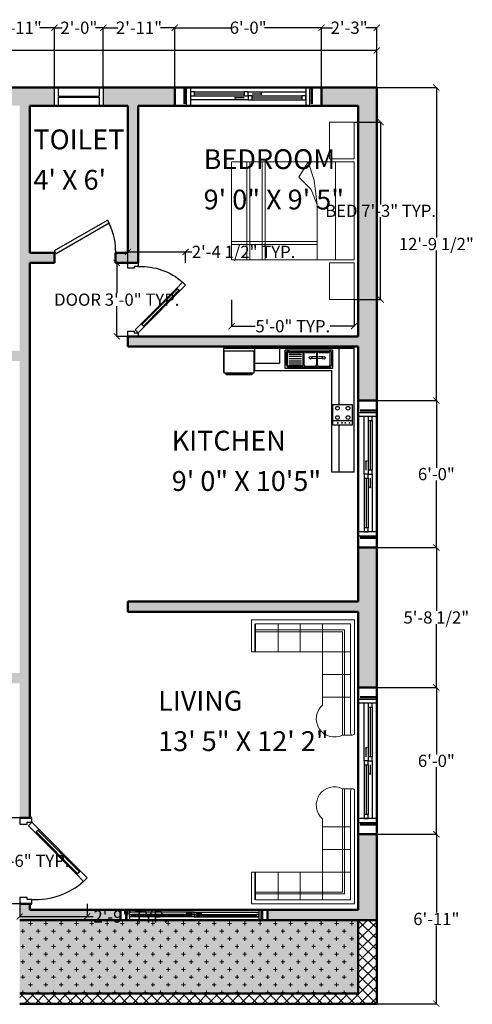
# Model space of a CAD drawing. Units: inches. Extents: x 2278 to 7495, y -71 to 1198.
# Tile 4 of 44: x 2542 to 2764, y 714 to 1197. Entities that reach past the tile are written whole.
import ezdxf

# ---------------------------------------------------------------- set-up
doc = ezdxf.new("R2010")
doc.units = ezdxf.units.IN
doc.header["$MEASUREMENT"] = 0
for name, color, linetype, lineweight in [('A-ANNO-DIMS', 2, 'Continuous', 18), ('A-AREA-IDEN', 3, 'Continuous', 18), ('A-Door', 3, 'Continuous', 25), ('A-FLOR-FIXT', 9, 'Continuous', 18), ('A-FURN', 8, 'Continuous', 18), ('A-Glaz', 4, 'Continuous', 25), ('A-Wall', 7, 'Continuous', 50), ('A-WALL-PATT', 8, 'Continuous', 18)]:
    doc.layers.add(name, color=color, linetype=linetype, lineweight=lineweight)
doc.layers.add('TEFRIŞ', color=11, linetype='Continuous')
doc.styles.get("Standard").update_dxf_attribs({"font": 'arial.ttf'})
doc.dimstyles.get("Standard").update_dxf_attribs({"dimtxt": 6, "dimasz": 3, "dimexe": 0.18, "dimexo": 0.0625, "dimgap": 0.09, "dimtad": 0, "dimtih": 1, "dimtoh": 1, "dimdec": 0, "dimzin": 0, "dimdsep": 46, "dimlunit": 3, "dimtxsty": 'Standard', "dimblk": 'ARCHTICK', "dimcen": 0.09, "dimadec": 0, "dimazin": 0, "dimtfac": 1, "dimtdec": 0, "dimtofl": 0, "dimtmove": 0, "dimatfit": 3, "dimfxl": 1, "dimtolj": 1, "dimtzin": 0, "dimarcsym": 0})

# ---------------------------------------------------------------- blocks, each defined once
blk = doc.blocks.new('A$C1DF4181C')
blk.add_lwpolyline([(120, 128), (460.7, 466.1), (432.5, 494.5), (91.8, 156.4)], close=True)
blk.add_arc((72.4, 128.7), 593.3, 357.23132, 41.49368)
at = {"layer": 'A-Door'}
for points in [[(517.5, 522.4), (460.7, 466.1), (432.5, 494.5), (489.3, 550.8)], [(35, 100), (0, 100), (0, 0), (50, 0), (50, 50), (50, 60), (35, 60)], [(63.2, 71.6), (120, 128), (91.8, 156.4), (35, 100)], [(665, 100), (665, 60), (650, 60), (650, 50), (650, 0), (700, 0), (700, 100)]]:
    blk.add_lwpolyline(points, close=True, dxfattribs=at)
at = {"layer": 'A-Glaz'}
blk.add_lwpolyline([(112.9, 135.1), (453.6, 473.2), (439.5, 487.4), (98.8, 149.3)], close=True, dxfattribs=at)
at = {"layer": 'A-Wall'}
for p, q in [((0, 0), (0, 100)), ((0, 100), (0, 0)), ((700, 0), (700, 100)), ((700, 0), (700, 100))]:
    blk.add_line(p, q, dxfattribs=at)
blk = doc.blocks.new('*U4')
for p, q in [((0, 0), (0, -6)), ((30, 0), (30, -6))]:
    blk.add_line(p, q)
blk.add_lwpolyline([(0, 0), (25.98, 15), (26.86, 13.48), (0.87, -1.52)], close=True)
blk.add_arc((0, 0), 30, 0, 30)
blk = doc.blocks.new('BED-160')
at = {"color": 0}
for p, q in [((-0.45, 2.35), (-0.45, 2.95)), ((-0.45, 2.95), (-0.05, 2.95)), ((-0.05, 2.95), (-0.05, 2.35)), ((-2.05, 2.3), (-0.05, 2.3)), ((-2.05, 0.7), (-2.05, 2.3)), ((-1.8, 0.7), (-1.8, 2.3)), ((-1.75, 0.7), (-1.75, 2.3)), ((-1.55, 0.7), (-1.55, 2.3)), ((-1.5, 0.7), (-1.5, 2.3)), ((-0.8, 2.3), (-0.95, 2.05)), ((-0.8, 2.3), (-0.7, 2)), ((-0.05, 2.35), (-0.45, 2.35)), ((-0.35, 0.7), (-0.35, 2.3)), ((-0.05, 2.3), (-0.05, 0.7)), ((-0.95, 2.05), (-0.75, 1.85)), ((-0.7, 2), (-0.65, 1.6)), ((-0.75, 1.85), (-0.65, 1.6)), ((-0.65, 1.6), (-0.65, 0.7)), ((-0.65, 1), (-2.05, 1)), ((-0.65, 0.95), (-2.05, 0.95)), ((-0.05, 0.7), (-2.05, 0.7)), ((-0.45, 0.65), (-0.05, 0.65)), ((-0.45, 0.05), (-0.45, 0.65)), ((-0.05, 0.65), (-0.05, 0.05)), ((-0.05, 0.05), (-0.45, 0.05))]:
    blk.add_line(p, q, dxfattribs=at)
blk = doc.blocks.new('A$C008029BD')
at = {"layer": 'TEFRIŞ', "ltscale": 0.05}
for p, q in [((0, 0), (0, -3.55)), ((3.37, 0), (0, 0)), ((3.37, 0), (3.37, -0.6)), ((1.522, -0.4), (0, -0.4)), ((3.37, -0.4), (2.083, -0.4)), ((0.05, -0.581), (0.05, -1.869)), ((0.05, -0.581), (0.55, -0.581)), ((0.086, -1.773), (0.086, -0.677)), ((0.096, -0.617), (0.454, -0.617)), ((0.099, -0.659), (0.457, -0.659)), ((0.113, -0.954), (0.113, -0.695)), ((0.493, -0.695), (0.493, -0.954)), ((0.514, -0.677), (0.514, -1.773)), ((0.55, -0.581), (0.55, -1.869)), ((0.6, -2.71), (0.6, -0.6)), ((3.37, -0.6), (0.6, -0.6)), ((0.096, -1.024), (0.454, -1.024)), ((0.457, -0.99), (0.099, -0.99)), ((0.11, -1.319), (0.11, -1.06)), ((0.228, -1.02), (0.227, -1.159)), ((0.23, -0.846), (0.229, -0.967)), ((0.28, -0.846), (0.277, -1.158)), ((0.49, -1.06), (0.49, -1.319)), ((0.454, -1.355), (0.096, -1.355)), ((0.096, -1.391), (0.454, -1.391)), ((0.11, -1.773), (0.11, -1.427)), ((0.154, -1.773), (0.154, -1.427)), ((0.214, -1.773), (0.214, -1.427)), ((0.274, -1.773), (0.274, -1.427)), ((0.334, -1.773), (0.334, -1.427)), ((0.39, -1.773), (0.39, -1.427)), ((0.444, -1.773), (0.444, -1.427)), ((0.49, -1.427), (0.49, -1.773)), ((0.55, -1.869), (0.05, -1.869)), ((0.454, -1.809), (0.096, -1.809)), ((0.454, -1.833), (0.096, -1.833)), ((0, -2.025), (0.4, -2.025)), ((0.4, -2.71), (0.4, -2.025)), ((0, -2.71), (0.6, -2.71)), ((0, -3.55), (0.65, -3.55))]:
    blk.add_line(p, q, dxfattribs=at)
at = {"layer": 'TEFRIŞ'}
blk.add_line((1.969, -0.05), (1.969, -0.572), dxfattribs=at)
at = {"layer": 'TEFRIŞ', "ltscale": 0.05}
for points in [[(1.522, -0.05), (2.083, -0.05), (2.083, -0.572), (1.522, -0.572)], [(0.67, -2.73), (0.67, -3.53), (0.07, -3.53), (0.07, -2.73)], [(0.72, -2.78), (0.72, -3.48), (0.67, -3.48), (0.67, -2.78)]]:
    blk.add_lwpolyline(points, close=True, dxfattribs=at)
at = {"layer": 'TEFRIŞ', "const_width": 0.025}
for points in [[(2.014, -0.123, 1), (2.039, -0.123, 1)], [(2.014, -0.236, 1), (2.039, -0.236, 1)], [(2.014, -0.327, 1), (2.039, -0.327, 1)], [(2.014, -0.44, 1), (2.039, -0.44, 1)]]:
    blk.add_lwpolyline(points, format="xyb", close=True, dxfattribs=at)
at = {"layer": 'TEFRIŞ', "ltscale": 0.05}
for centre, radius in [((1.628, -0.164), 0.0505), ((1.628, -0.45), 0.0505), ((0.255, -0.82), 0.036), ((0.252, -1.184), 0.036)]:
    blk.add_circle(centre, radius, dxfattribs=at)
at = {"layer": 'TEFRIŞ'}
for centre in [(1.88, -0.164), (1.88, -0.45)]:
    blk.add_circle(centre, 0.0505, dxfattribs=at)
at = {"layer": 'TEFRIŞ', "ltscale": 0.05}
for centre, radius, start, end in [((0.108, -0.649), 0.0351, 110.4976, 230.5777), ((0.118, -0.673), 0.023, 143.9853, 258.5157), ((0.454, -0.677), 0.06, 0, 90), ((0.457, -0.695), 0.036, 0, 90), ((0.115, -1.038), 0.023, 143.9853, 258.5157), ((0.118, -0.976), 0.023, 101.4843, 216.0147), ((0.454, -1.06), 0.036, 0, 90), ((0.457, -0.954), 0.036, 270, 0), ((0.115, -1.341), 0.023, 101.4843, 216.0147), ((0.454, -1.319), 0.036, 270, 0), ((0.115, -1.405), 0.023, 143.9853, 258.5157), ((0.454, -1.427), 0.036, 0, 90), ((0.108, -1.801), 0.0351, 129.4223, 249.5024), ((0.115, -1.796), 0.023, 101.4843, 216.0147), ((0.454, -1.773), 0.06, 270, 0), ((0.454, -1.773), 0.036, 270, 0)]:
    blk.add_arc(centre, radius, start, end, dxfattribs=at)
blk = doc.blocks.new('_ArchTick')
at = {"color": 0, "linetype": 'ByBlock', "const_width": 0.15}
blk.add_lwpolyline([(-0.5, -0.5), (0.5, 0.5)], dxfattribs=at)
blk = doc.blocks.new('*D18')
at = {"layer": 'A-ANNO-DIMS', "color": 0, "lineweight": -2, "transparency": 16777216}
for p, q in [((2313.87, 1163.53), (2313.87, 1181.72)), ((2313.87, 1181.54), (2504.98, 1181.54)), ((2716.87, 1181.54), (2525.76, 1181.54)), ((2716.87, 1163.53), (2716.87, 1181.72))]:
    blk.add_line(p, q, dxfattribs=at)
at = {"layer": 'Defpoints', "color": 0, "transparency": 16777216}
for p in [(2716.87, 1181.54), (2313.87, 1163.47), (2716.87, 1163.47)]:
    blk.add_point(p, dxfattribs=at)
at = {"layer": 'A-ANNO-DIMS', "color": 0, "lineweight": -2, "transparency": 16777216, "xscale": 3, "yscale": 3, "zscale": 3, "rotation": 180}
blk.add_blockref('_ArchTick', (2313.87, 1181.54), dxfattribs=at)
at = {"layer": 'A-ANNO-DIMS', "color": 0, "lineweight": -2, "transparency": 16777216, "xscale": 3, "yscale": 3, "zscale": 3}
blk.add_blockref('_ArchTick', (2716.87, 1181.54), dxfattribs=at)
at = {"layer": 'A-ANNO-DIMS', "color": 0, "transparency": 16777216, "insert": (2515.37, 1181.54), "char_height": 6, "attachment_point": 5}
blk.add_mtext('\\A1;33\'-7"', dxfattribs=at)
blk = doc.blocks.new('*D43')
at = {"layer": 'A-ANNO-DIMS', "color": 0, "lineweight": -2, "transparency": 16777216}
for p, q in [((2541.81, 805.47), (2535.39, 805.47)), ((2535.57, 805.47), (2535.57, 787.66)), ((2535.57, 763.47), (2535.57, 781.27)), ((2541.81, 763.47), (2535.39, 763.47))]:
    blk.add_line(p, q, dxfattribs=at)
at = {"layer": 'Defpoints', "color": 0, "transparency": 16777216}
for p in [(2541.87, 805.47), (2535.57, 763.47), (2541.87, 763.47)]:
    blk.add_point(p, dxfattribs=at)
at = {"layer": 'A-ANNO-DIMS', "color": 0, "lineweight": -2, "transparency": 16777216, "xscale": 3, "yscale": 3, "zscale": 3}
for p, rotation in [((2535.57, 805.47), 90), ((2535.57, 763.47), 270)]:
    blk.add_blockref('_ArchTick', p, dxfattribs=dict(at, rotation=rotation))
at = {"layer": 'A-ANNO-DIMS', "color": 0, "transparency": 16777216, "insert": (2535.57, 784.47), "char_height": 6, "attachment_point": 5}
blk.add_mtext('\\A1;DOOR 3\'-6" TYP.', dxfattribs=at)
blk = doc.blocks.new('*D44')
at = {"layer": 'A-ANNO-DIMS', "color": 0, "lineweight": -2, "transparency": 16777216}
for p, q in [((2541.87, 763.4), (2541.87, 756.99)), ((2574.92, 763.4), (2574.92, 756.99)), ((2541.87, 757.17), (2574.92, 757.17)), ((2574.92, 757.17), (2577.92, 757.17))]:
    blk.add_line(p, q, dxfattribs=at)
at = {"layer": 'Defpoints', "color": 0, "transparency": 16777216}
for p in [(2541.87, 763.47), (2574.92, 763.47), (2574.92, 757.17)]:
    blk.add_point(p, dxfattribs=at)
at = {"layer": 'A-ANNO-DIMS', "color": 0, "lineweight": -2, "transparency": 16777216, "xscale": 3, "yscale": 3, "zscale": 3, "rotation": 180}
blk.add_blockref('_ArchTick', (2541.87, 757.17), dxfattribs=at)
at = {"layer": 'A-ANNO-DIMS', "color": 0, "lineweight": -2, "transparency": 16777216, "xscale": 3, "yscale": 3, "zscale": 3}
blk.add_blockref('_ArchTick', (2574.92, 757.17), dxfattribs=at)
at = {"layer": 'A-ANNO-DIMS', "color": 0, "transparency": 16777216, "insert": (2596.35, 757.17), "char_height": 6, "attachment_point": 5}
blk.add_mtext('\\A1;2\'-9" TYP.', dxfattribs=at)
blk = doc.blocks.new('*D45')
at = {"layer": 'A-ANNO-DIMS', "color": 0, "lineweight": -2, "transparency": 16777216}
for p, q in [((2594.81, 1077.47), (2589.29, 1077.47)), ((2589.47, 1077.47), (2589.47, 1062.66)), ((2589.47, 1041.47), (2589.47, 1056.27)), ((2594.81, 1041.47), (2589.29, 1041.47))]:
    blk.add_line(p, q, dxfattribs=at)
at = {"layer": 'Defpoints', "color": 0, "transparency": 16777216}
for p in [(2589.47, 1077.47), (2594.87, 1077.47), (2594.87, 1041.47)]:
    blk.add_point(p, dxfattribs=at)
at = {"layer": 'A-ANNO-DIMS', "color": 0, "lineweight": -2, "transparency": 16777216, "xscale": 3, "yscale": 3, "zscale": 3}
for p, rotation in [((2589.47, 1077.47), 90), ((2589.47, 1041.47), 270)]:
    blk.add_blockref('_ArchTick', p, dxfattribs=dict(at, rotation=rotation))
at = {"layer": 'A-ANNO-DIMS', "color": 0, "transparency": 16777216, "insert": (2589.47, 1059.47), "char_height": 6, "attachment_point": 5}
blk.add_mtext('\\A1;DOOR 3\'-0" TYP.', dxfattribs=at)
blk = doc.blocks.new('*D46')
at = {"layer": 'A-ANNO-DIMS', "color": 0, "lineweight": -2, "transparency": 16777216}
for p, q in [((2594.87, 1077.53), (2594.87, 1083.05)), ((2594.87, 1082.87), (2623.2, 1082.87)), ((2623.2, 1077.53), (2623.2, 1083.05)), ((2623.2, 1082.87), (2626.2, 1082.87))]:
    blk.add_line(p, q, dxfattribs=at)
at = {"layer": 'Defpoints', "color": 0, "transparency": 16777216}
for p in [(2623.2, 1082.87), (2594.87, 1077.47), (2623.2, 1077.47)]:
    blk.add_point(p, dxfattribs=at)
at = {"layer": 'A-ANNO-DIMS', "color": 0, "lineweight": -2, "transparency": 16777216, "xscale": 3, "yscale": 3, "zscale": 3, "rotation": 180}
blk.add_blockref('_ArchTick', (2594.87, 1082.87), dxfattribs=at)
at = {"layer": 'A-ANNO-DIMS', "color": 0, "lineweight": -2, "transparency": 16777216, "xscale": 3, "yscale": 3, "zscale": 3}
blk.add_blockref('_ArchTick', (2623.2, 1082.87), dxfattribs=at)
at = {"layer": 'A-ANNO-DIMS', "color": 0, "transparency": 16777216, "insert": (2651.62, 1082.87), "char_height": 6, "attachment_point": 5}
blk.add_mtext('\\A1;2\'-4 1/2" TYP.', dxfattribs=at)
blk = doc.blocks.new('*D49')
at = {"layer": 'A-ANNO-DIMS', "color": 0, "lineweight": -2, "transparency": 16777216}
for p, q in [((2705.82, 1146.5), (2718.99, 1146.5)), ((2718.81, 1146.5), (2718.81, 1106.15)), ((2718.81, 1059.5), (2718.81, 1099.84)), ((2705.82, 1059.5), (2718.99, 1059.5))]:
    blk.add_line(p, q, dxfattribs=at)
at = {"layer": 'Defpoints', "color": 0, "transparency": 16777216}
for p in [(2705.76, 1146.5), (2718.81, 1146.5), (2705.76, 1059.5)]:
    blk.add_point(p, dxfattribs=at)
at = {"layer": 'A-ANNO-DIMS', "color": 0, "lineweight": -2, "transparency": 16777216, "xscale": 3, "yscale": 3, "zscale": 3}
for p, rotation in [((2718.81, 1146.5), 90), ((2718.81, 1059.5), 270)]:
    blk.add_blockref('_ArchTick', p, dxfattribs=dict(at, rotation=rotation))
at = {"layer": 'A-ANNO-DIMS', "color": 0, "transparency": 16777216, "insert": (2718.81, 1103), "char_height": 6, "attachment_point": 5}
blk.add_mtext('\\A1;BED 7\'-3" TYP.', dxfattribs=at)
blk = doc.blocks.new('*D50')
at = {"layer": 'A-ANNO-DIMS', "color": 0, "lineweight": -2, "transparency": 16777216}
for p, q in [((2645.76, 1059.43), (2645.76, 1046.27)), ((2705.76, 1059.43), (2705.76, 1046.27)), ((2645.76, 1046.45), (2657.38, 1046.45)), ((2705.76, 1046.45), (2694.14, 1046.45))]:
    blk.add_line(p, q, dxfattribs=at)
at = {"layer": 'Defpoints', "color": 0, "transparency": 16777216}
for p in [(2645.76, 1059.5), (2705.76, 1059.5), (2705.76, 1046.45)]:
    blk.add_point(p, dxfattribs=at)
at = {"layer": 'A-ANNO-DIMS', "color": 0, "lineweight": -2, "transparency": 16777216, "xscale": 3, "yscale": 3, "zscale": 3, "rotation": 180}
blk.add_blockref('_ArchTick', (2645.76, 1046.45), dxfattribs=at)
at = {"layer": 'A-ANNO-DIMS', "color": 0, "lineweight": -2, "transparency": 16777216, "xscale": 3, "yscale": 3, "zscale": 3}
blk.add_blockref('_ArchTick', (2705.76, 1046.45), dxfattribs=at)
at = {"layer": 'A-ANNO-DIMS', "color": 0, "transparency": 16777216, "insert": (2675.76, 1046.45), "char_height": 6, "attachment_point": 5}
blk.add_mtext('\\A1;5\'-0" TYP.', dxfattribs=at)
blk = doc.blocks.new('*D65')
at = {"layer": 'A-ANNO-DIMS', "color": 0, "lineweight": -2, "transparency": 16777216}
for p, q in [((2523.87, 1163.53), (2523.87, 1192.9)), ((2523.87, 1192.72), (2530.92, 1192.72)), ((2558.87, 1192.72), (2551.82, 1192.72)), ((2558.87, 1163.53), (2558.87, 1192.9))]:
    blk.add_line(p, q, dxfattribs=at)
at = {"layer": 'Defpoints', "color": 0, "transparency": 16777216}
for p in [(2558.87, 1192.72), (2523.87, 1163.47), (2558.87, 1163.47)]:
    blk.add_point(p, dxfattribs=at)
at = {"layer": 'A-ANNO-DIMS', "color": 0, "lineweight": -2, "transparency": 16777216, "xscale": 3, "yscale": 3, "zscale": 3, "rotation": 180}
blk.add_blockref('_ArchTick', (2523.87, 1192.72), dxfattribs=at)
at = {"layer": 'A-ANNO-DIMS', "color": 0, "lineweight": -2, "transparency": 16777216, "xscale": 3, "yscale": 3, "zscale": 3}
blk.add_blockref('_ArchTick', (2558.87, 1192.72), dxfattribs=at)
at = {"layer": 'A-ANNO-DIMS', "color": 0, "transparency": 16777216, "insert": (2541.37, 1192.72), "char_height": 6, "attachment_point": 5}
blk.add_mtext('\\A1;2\'-11"', dxfattribs=at)
blk = doc.blocks.new('*D66')
at = {"layer": 'A-ANNO-DIMS', "color": 0, "lineweight": -2, "transparency": 16777216}
for p, q in [((2558.87, 1163.53), (2558.87, 1192.9)), ((2558.87, 1192.72), (2562.75, 1192.72)), ((2582.87, 1192.72), (2578.99, 1192.72)), ((2582.87, 1163.53), (2582.87, 1192.9))]:
    blk.add_line(p, q, dxfattribs=at)
at = {"layer": 'Defpoints', "color": 0, "transparency": 16777216}
for p in [(2582.87, 1192.72), (2558.87, 1163.47), (2582.87, 1163.47)]:
    blk.add_point(p, dxfattribs=at)
at = {"layer": 'A-ANNO-DIMS', "color": 0, "lineweight": -2, "transparency": 16777216, "xscale": 3, "yscale": 3, "zscale": 3, "rotation": 180}
blk.add_blockref('_ArchTick', (2558.87, 1192.72), dxfattribs=at)
at = {"layer": 'A-ANNO-DIMS', "color": 0, "lineweight": -2, "transparency": 16777216, "xscale": 3, "yscale": 3, "zscale": 3}
blk.add_blockref('_ArchTick', (2582.87, 1192.72), dxfattribs=at)
at = {"layer": 'A-ANNO-DIMS', "color": 0, "transparency": 16777216, "insert": (2570.87, 1192.72), "char_height": 6, "attachment_point": 5}
blk.add_mtext('\\A1;2\'-0"', dxfattribs=at)
blk = doc.blocks.new('*D67')
at = {"layer": 'A-ANNO-DIMS', "color": 0, "lineweight": -2, "transparency": 16777216}
for p, q in [((2582.87, 1163.53), (2582.87, 1192.9)), ((2582.87, 1192.72), (2589.92, 1192.72)), ((2617.87, 1192.72), (2610.82, 1192.72)), ((2617.87, 1163.53), (2617.87, 1192.9))]:
    blk.add_line(p, q, dxfattribs=at)
at = {"layer": 'Defpoints', "color": 0, "transparency": 16777216}
for p in [(2617.87, 1192.72), (2582.87, 1163.47), (2617.87, 1163.47)]:
    blk.add_point(p, dxfattribs=at)
at = {"layer": 'A-ANNO-DIMS', "color": 0, "lineweight": -2, "transparency": 16777216, "xscale": 3, "yscale": 3, "zscale": 3, "rotation": 180}
blk.add_blockref('_ArchTick', (2582.87, 1192.72), dxfattribs=at)
at = {"layer": 'A-ANNO-DIMS', "color": 0, "lineweight": -2, "transparency": 16777216, "xscale": 3, "yscale": 3, "zscale": 3}
blk.add_blockref('_ArchTick', (2617.87, 1192.72), dxfattribs=at)
at = {"layer": 'A-ANNO-DIMS', "color": 0, "transparency": 16777216, "insert": (2600.37, 1192.72), "char_height": 6, "attachment_point": 5}
blk.add_mtext('\\A1;2\'-11"', dxfattribs=at)
blk = doc.blocks.new('*D68')
at = {"layer": 'A-ANNO-DIMS', "color": 0, "lineweight": -2, "transparency": 16777216}
for p, q in [((2617.87, 1163.53), (2617.87, 1192.9)), ((2617.87, 1192.72), (2645.79, 1192.72)), ((2689.87, 1192.72), (2661.95, 1192.72)), ((2689.87, 1163.53), (2689.87, 1192.9))]:
    blk.add_line(p, q, dxfattribs=at)
at = {"layer": 'Defpoints', "color": 0, "transparency": 16777216}
for p in [(2689.87, 1192.72), (2617.87, 1163.47), (2689.87, 1163.47)]:
    blk.add_point(p, dxfattribs=at)
at = {"layer": 'A-ANNO-DIMS', "color": 0, "lineweight": -2, "transparency": 16777216, "xscale": 3, "yscale": 3, "zscale": 3, "rotation": 180}
blk.add_blockref('_ArchTick', (2617.87, 1192.72), dxfattribs=at)
at = {"layer": 'A-ANNO-DIMS', "color": 0, "lineweight": -2, "transparency": 16777216, "xscale": 3, "yscale": 3, "zscale": 3}
blk.add_blockref('_ArchTick', (2689.87, 1192.72), dxfattribs=at)
at = {"layer": 'A-ANNO-DIMS', "color": 0, "transparency": 16777216, "insert": (2653.87, 1192.72), "char_height": 6, "attachment_point": 5}
blk.add_mtext('\\A1;6\'-0"', dxfattribs=at)
blk = doc.blocks.new('*D69')
at = {"layer": 'A-ANNO-DIMS', "color": 0, "lineweight": -2, "transparency": 16777216}
for p, q in [((2689.87, 1163.53), (2689.87, 1192.9)), ((2689.87, 1192.72), (2695.25, 1192.72)), ((2716.87, 1192.72), (2711.49, 1192.72)), ((2716.87, 1163.53), (2716.87, 1192.9))]:
    blk.add_line(p, q, dxfattribs=at)
at = {"layer": 'Defpoints', "color": 0, "transparency": 16777216}
for p in [(2716.87, 1192.72), (2689.87, 1163.47), (2716.87, 1163.47)]:
    blk.add_point(p, dxfattribs=at)
at = {"layer": 'A-ANNO-DIMS', "color": 0, "lineweight": -2, "transparency": 16777216, "xscale": 3, "yscale": 3, "zscale": 3, "rotation": 180}
blk.add_blockref('_ArchTick', (2689.87, 1192.72), dxfattribs=at)
at = {"layer": 'A-ANNO-DIMS', "color": 0, "lineweight": -2, "transparency": 16777216, "xscale": 3, "yscale": 3, "zscale": 3}
blk.add_blockref('_ArchTick', (2716.87, 1192.72), dxfattribs=at)
at = {"layer": 'A-ANNO-DIMS', "color": 0, "transparency": 16777216, "insert": (2703.37, 1192.72), "char_height": 6, "attachment_point": 5}
blk.add_mtext('\\A1;2\'-3"', dxfattribs=at)
blk = doc.blocks.new('*D70')
at = {"layer": 'A-ANNO-DIMS', "color": 0, "lineweight": -2, "transparency": 16777216}
for p, q in [((2716.93, 1163.47), (2746.3, 1163.47)), ((2746.12, 1163.47), (2746.12, 1089.91)), ((2746.12, 1009.97), (2746.12, 1083.52)), ((2716.93, 1009.97), (2746.3, 1009.97))]:
    blk.add_line(p, q, dxfattribs=at)
at = {"layer": 'Defpoints', "color": 0, "transparency": 16777216}
for p in [(2716.87, 1163.47), (2716.87, 1009.97), (2746.12, 1009.97)]:
    blk.add_point(p, dxfattribs=at)
at = {"layer": 'A-ANNO-DIMS', "color": 0, "lineweight": -2, "transparency": 16777216, "xscale": 3, "yscale": 3, "zscale": 3}
for p, rotation in [((2746.12, 1163.47), 90), ((2746.12, 1009.97), 270)]:
    blk.add_blockref('_ArchTick', p, dxfattribs=dict(at, rotation=rotation))
at = {"layer": 'A-ANNO-DIMS', "color": 0, "transparency": 16777216, "insert": (2746.12, 1086.72), "char_height": 6, "attachment_point": 5}
blk.add_mtext('\\A1;12\'-9 1/2"', dxfattribs=at)
blk = doc.blocks.new('*D71')
at = {"layer": 'A-ANNO-DIMS', "color": 0, "lineweight": -2, "transparency": 16777216}
for p, q in [((2716.93, 1009.97), (2746.3, 1009.97)), ((2746.12, 1009.97), (2746.12, 977.12)), ((2746.12, 937.97), (2746.12, 970.81)), ((2716.93, 937.97), (2746.3, 937.97))]:
    blk.add_line(p, q, dxfattribs=at)
at = {"layer": 'Defpoints', "color": 0, "transparency": 16777216}
for p in [(2716.87, 1009.97), (2716.87, 937.97), (2746.12, 937.97)]:
    blk.add_point(p, dxfattribs=at)
at = {"layer": 'A-ANNO-DIMS', "color": 0, "lineweight": -2, "transparency": 16777216, "xscale": 3, "yscale": 3, "zscale": 3}
for p, rotation in [((2746.12, 1009.97), 90), ((2746.12, 937.97), 270)]:
    blk.add_blockref('_ArchTick', p, dxfattribs=dict(at, rotation=rotation))
at = {"layer": 'A-ANNO-DIMS', "color": 0, "transparency": 16777216, "insert": (2746.12, 973.97), "char_height": 6, "attachment_point": 5}
blk.add_mtext('\\A1;6\'-0"', dxfattribs=at)
blk = doc.blocks.new('*D72')
at = {"layer": 'A-ANNO-DIMS', "color": 0, "lineweight": -2, "transparency": 16777216}
for p, q in [((2716.93, 937.97), (2746.3, 937.97)), ((2746.12, 937.97), (2746.12, 906.91)), ((2746.12, 869.47), (2746.12, 900.52)), ((2716.93, 869.47), (2746.3, 869.47))]:
    blk.add_line(p, q, dxfattribs=at)
at = {"layer": 'Defpoints', "color": 0, "transparency": 16777216}
for p in [(2716.87, 937.97), (2716.87, 869.47), (2746.12, 869.47)]:
    blk.add_point(p, dxfattribs=at)
at = {"layer": 'A-ANNO-DIMS', "color": 0, "lineweight": -2, "transparency": 16777216, "xscale": 3, "yscale": 3, "zscale": 3}
for p, rotation in [((2746.12, 937.97), 90), ((2746.12, 869.47), 270)]:
    blk.add_blockref('_ArchTick', p, dxfattribs=dict(at, rotation=rotation))
at = {"layer": 'A-ANNO-DIMS', "color": 0, "transparency": 16777216, "insert": (2746.12, 903.72), "char_height": 6, "attachment_point": 5}
blk.add_mtext('\\A1;5\'-8 1/2"', dxfattribs=at)
blk = doc.blocks.new('*D73')
at = {"layer": 'A-ANNO-DIMS', "color": 0, "lineweight": -2, "transparency": 16777216}
for p, q in [((2716.93, 869.47), (2746.3, 869.47)), ((2746.12, 869.47), (2746.12, 836.62)), ((2746.12, 797.47), (2746.12, 830.31)), ((2716.93, 797.47), (2746.3, 797.47))]:
    blk.add_line(p, q, dxfattribs=at)
at = {"layer": 'Defpoints', "color": 0, "transparency": 16777216}
for p in [(2716.87, 869.47), (2716.87, 797.47), (2746.12, 797.47)]:
    blk.add_point(p, dxfattribs=at)
at = {"layer": 'A-ANNO-DIMS', "color": 0, "lineweight": -2, "transparency": 16777216, "xscale": 3, "yscale": 3, "zscale": 3}
for p, rotation in [((2746.12, 869.47), 90), ((2746.12, 797.47), 270)]:
    blk.add_blockref('_ArchTick', p, dxfattribs=dict(at, rotation=rotation))
at = {"layer": 'A-ANNO-DIMS', "color": 0, "transparency": 16777216, "insert": (2746.12, 833.47), "char_height": 6, "attachment_point": 5}
blk.add_mtext('\\A1;6\'-0"', dxfattribs=at)
blk = doc.blocks.new('*D74')
at = {"layer": 'A-ANNO-DIMS', "color": 0, "lineweight": -2, "transparency": 16777216}
for p, q in [((2716.93, 797.47), (2746.3, 797.47)), ((2746.12, 797.47), (2746.12, 759.12)), ((2746.12, 714.47), (2746.12, 752.81)), ((2716.93, 714.47), (2746.3, 714.47))]:
    blk.add_line(p, q, dxfattribs=at)
at = {"layer": 'Defpoints', "color": 0, "transparency": 16777216}
for p in [(2716.87, 797.47), (2716.87, 714.47), (2746.12, 714.47)]:
    blk.add_point(p, dxfattribs=at)
at = {"layer": 'A-ANNO-DIMS', "color": 0, "lineweight": -2, "transparency": 16777216, "xscale": 3, "yscale": 3, "zscale": 3}
for p, rotation in [((2746.12, 797.47), 90), ((2746.12, 714.47), 270)]:
    blk.add_blockref('_ArchTick', p, dxfattribs=dict(at, rotation=rotation))
at = {"layer": 'A-ANNO-DIMS', "color": 0, "transparency": 16777216, "insert": (2746.12, 755.97), "char_height": 6, "attachment_point": 5}
blk.add_mtext('\\A1;6\'-11"', dxfattribs=at)

msp = doc.modelspace()

# ---------------------------------------------------------------- hatches: boundary and pattern name
at = {"layer": 'A-WALL-PATT'}
h = msp.add_hatch(dxfattribs=at)
h.set_pattern_fill('ANSI36', color=256, scale=30)
h.paths.add_polyline_path([(2343.12, 957.47), (2322.87, 957.47), (2322.87, 1029.47), (2351.87, 1029.47), (2351.87, 1034.47), (2322.87, 1034.47), (2322.87, 1154.47), (2339.87, 1154.47), (2339.87, 1163.47), (2313.87, 1163.47), (2313.87, 710.47), (2445.87, 710.47), (2445.87, 719.47), (2322.87, 719.47), (2322.87, 807.47), (2404.87, 807.47), (2404.87, 812.47), (2392.87, 812.47), (2392.87, 881.47), (2387.87, 881.47), (2387.87, 812.47), (2322.87, 812.47), (2322.87, 911.47), (2345.87, 911.47), (2345.87, 916.47), (2322.87, 916.47), (2322.87, 952.47), (2343.12, 952.47)])
h.paths.add_polyline_path([(2451.87, 1163.47), (2411.87, 1163.47), (2411.87, 1154.47), (2428.87, 1154.47), (2428.87, 1034.47), (2428.87, 1029.47), (2433.87, 1029.47), (2433.87, 1154.47), (2451.87, 1154.47)])
h.paths.add_polyline_path([(2558.87, 1163.47), (2523.87, 1163.47), (2523.87, 1154.47), (2541.87, 1154.47), (2541.87, 1034.47), (2475.87, 1034.47), (2475.87, 1029.47), (2541.87, 1029.47), (2541.87, 943.47), (2541.87, 940.13), (2541.87, 876.47), (2493.87, 876.47), (2493.87, 943.47), (2488.87, 943.47), (2488.87, 871.47), (2488.87, 865.74), (2493.88, 865.74), (2493.88, 871.47), (2541.87, 871.47), (2541.87, 805.47), (2546.87, 805.47), (2546.87, 1077.47), (2558.87, 1077.47), (2558.87, 1082.47), (2546.87, 1082.47), (2546.87, 1154.47), (2558.87, 1154.47)])
h.paths.add_polyline_path([(2716.87, 937.97), (2707.87, 937.97), (2707.87, 911.47), (2594.87, 911.47), (2594.87, 906.47), (2707.87, 906.47), (2707.87, 869.47), (2716.87, 869.47)])
h.paths.add_polyline_path([(2716.87, 1163.47), (2689.87, 1163.47), (2689.87, 1154.47), (2707.87, 1154.47), (2707.87, 1041.47), (2594.87, 1041.47), (2594.87, 1036.47), (2707.87, 1036.47), (2707.87, 1009.97), (2716.87, 1009.97)])
h.paths.add_polyline_path([(2617.87, 1163.47), (2582.87, 1163.47), (2582.87, 1154.47), (2594.87, 1154.47), (2594.87, 1082.47), (2588.87, 1082.47), (2588.87, 1077.47), (2599.87, 1077.47), (2599.87, 1154.47), (2617.87, 1154.47)])
h.paths.add_polyline_path([(2716.87, 797.47), (2707.87, 797.47), (2707.87, 760.47), (2663.37, 760.47), (2663.37, 755.47), (2716.87, 755.47)])
h.paths.add_polyline_path([(2591.37, 760.47), (2546.87, 760.47), (2546.87, 763.47), (2541.87, 763.47), (2541.87, 755.47), (2591.37, 755.47)])
h = msp.add_hatch(dxfattribs=at)
h.set_pattern_fill('ANSI37', color=256, scale=30)
h.paths.add_polyline_path([(2716.87, 755.47), (2707.87, 755.47), (2707.87, 719.47), (2541.87, 719.47), (2541.87, 714.47), (2716.87, 714.47)])
at = {"layer": 'A-WALL-PATT', "transparency": 33554562}
h = msp.add_hatch(color=256, dxfattribs=at)
h.dxf.hatch_style = 1
h.paths.add_polyline_path([(2707.87, 755.47), (2541.87, 755.47), (2541.87, 719.47), (2707.87, 719.47)])
h = msp.add_hatch(dxfattribs=at)
h.set_pattern_fill('CROSS', color=256, scale=15)
h.paths.add_polyline_path([(2707.87, 755.47), (2541.87, 755.47), (2541.87, 719.47), (2707.87, 719.47)])

# ---------------------------------------------------------------- linework, layer by layer
at = {"layer": 'A-FURN'}
for p, q in [((2706.02, 902.55), (2655.5, 902.55)), ((2655.5, 902.55), (2655.5, 886.91)), ((2706.02, 847.04), (2706.02, 902.55)), ((2657.13, 900.59), (2657.13, 886.91)), ((2704.06, 900.59), (2657.45, 900.59)), ((2657.45, 900.59), (2657.45, 886.91)), ((2701.13, 897.66), (2657.45, 897.66)), ((2668.54, 900.59), (2668.54, 886.91)), ((2679.29, 900.59), (2679.29, 886.91)), ((2690.37, 900.59), (2690.37, 864.74)), ((2701.13, 846.06), (2701.13, 897.66)), ((2704.06, 847.04), (2704.06, 900.59)), ((2700.15, 896.68), (2657.45, 896.68)), ((2700.15, 846.06), (2700.15, 896.68)), ((2690.37, 889.51), (2690.37, 864.74)), ((2655.5, 886.91), (2704.06, 886.91)), ((2690.37, 875.82), (2704.06, 875.82)), ((2690.37, 864.74), (2704.06, 864.74)), ((2690.37, 864.74), (2704.06, 864.74)), ((2690.37, 864.74), (2690.37, 860.83)), ((2705.04, 846.06), (2700.15, 846.06)), ((2700.15, 819.82), (2700.15, 769.19)), ((2705.04, 819.82), (2700.15, 819.82)), ((2701.13, 819.82), (2701.13, 768.22)), ((2704.06, 818.84), (2704.06, 765.28)), ((2706.02, 818.84), (2706.02, 763.33)), ((2690.37, 801.14), (2690.37, 805.05)), ((2690.37, 765.28), (2690.37, 801.14)), ((2690.37, 776.37), (2690.37, 801.14)), ((2690.37, 801.14), (2704.06, 801.14)), ((2690.37, 801.14), (2704.06, 801.14)), ((2690.37, 790.05), (2704.06, 790.05)), ((2655.5, 778.97), (2704.06, 778.97)), ((2655.5, 763.33), (2655.5, 778.97)), ((2657.13, 765.28), (2657.13, 778.97)), ((2657.45, 765.28), (2657.45, 778.97)), ((2668.54, 765.28), (2668.54, 778.97)), ((2679.29, 765.28), (2679.29, 778.97)), ((2700.15, 769.19), (2657.45, 769.19)), ((2701.13, 768.22), (2657.45, 768.22)), ((2706.02, 763.33), (2655.5, 763.33)), ((2704.06, 765.28), (2657.45, 765.28))]:
    msp.add_line(p, q, dxfattribs=at)
for centre, radius, start, end in [((2696.18, 854.05), 8.93, 130.6021, 296.4078), ((2705.04, 847.04), 0.978, 180, 0), ((2696.18, 811.82), 8.93, 63.5922, 229.3979), ((2705.04, 818.84), 0.978, 0, 180)]:
    msp.add_arc(centre, radius, start, end, dxfattribs=at)
at = {"layer": 'A-Glaz'}
for p, q in [((2558.87, 1163.47), (2582.87, 1163.47)), ((2558.87, 1154.47), (2558.87, 1163.47)), ((2560.87, 1159.17), (2560.87, 1163.47)), ((2580.87, 1163.47), (2580.87, 1159.17)), ((2582.87, 1163.47), (2582.87, 1154.47)), ((2625.57, 1163.47), (2682.17, 1163.47)), ((2560.87, 1159.17), (2580.87, 1159.17)), ((2560.87, 1154.47), (2560.87, 1158.77)), ((2560.87, 1158.77), (2580.87, 1158.77)), ((2580.87, 1158.77), (2580.87, 1154.47)), ((2627.52, 1161.3), (2651.92, 1161.3)), ((2627.52, 1160.32), (2651.92, 1160.32)), ((2627.52, 1159.35), (2651.92, 1159.35)), ((2651.92, 1158.37), (2647.73, 1158.37)), ((2653.87, 1161.3), (2682.17, 1161.3)), ((2655.82, 1160.32), (2660.01, 1160.32)), ((2655.82, 1159.35), (2680.22, 1159.35)), ((2655.82, 1158.37), (2680.22, 1158.37)), ((2582.87, 1154.47), (2558.87, 1154.47)), ((2653.87, 1157.39), (2625.57, 1157.39)), ((2625.57, 1154.47), (2682.17, 1154.47)), ((2655.82, 1157.39), (2680.22, 1157.39)), ((2707.87, 1002.27), (2707.87, 945.67)), ((2710.8, 973.97), (2710.8, 1002.27)), ((2712.75, 1000.31), (2712.75, 975.92)), ((2713.73, 1000.31), (2713.73, 975.92)), ((2714.7, 1000.31), (2714.7, 975.92)), ((2716.87, 1002.27), (2716.87, 945.67)), ((2711.77, 975.92), (2711.77, 980.11)), ((2710.8, 972.01), (2710.8, 947.62)), ((2711.77, 972.01), (2711.77, 947.62)), ((2712.75, 972.01), (2712.75, 947.62)), ((2713.73, 972.01), (2713.73, 967.82)), ((2714.7, 973.97), (2714.7, 945.67)), ((2707.87, 861.77), (2707.87, 805.17)), ((2710.8, 833.47), (2710.8, 861.77)), ((2712.75, 859.81), (2712.75, 835.42)), ((2713.73, 859.81), (2713.73, 835.42)), ((2714.7, 859.81), (2714.7, 835.42)), ((2716.87, 861.77), (2716.87, 805.17)), ((2711.77, 835.42), (2711.77, 839.61)), ((2710.8, 831.51), (2710.8, 807.12)), ((2711.77, 831.51), (2711.77, 807.12)), ((2712.75, 831.51), (2712.75, 807.12)), ((2713.73, 831.51), (2713.73, 827.32)), ((2714.7, 833.47), (2714.7, 805.17)), ((2627.37, 760.47), (2595.65, 760.47)), ((2627.37, 759.26), (2595.65, 759.26)), ((2626.29, 758.18), (2596.73, 758.18)), ((2626.29, 757.64), (2596.73, 757.64)), ((2626.29, 758.72), (2623.96, 758.72)), ((2627.37, 760.47), (2659.09, 760.47)), ((2627.37, 759.26), (2659.09, 759.26)), ((2628.45, 758.72), (2630.78, 758.72)), ((2628.45, 758.18), (2658.01, 758.18)), ((2628.45, 757.64), (2658.01, 757.64)), ((2627.37, 755.47), (2595.65, 755.47)), ((2626.29, 757.09), (2596.73, 757.09)), ((2627.37, 755.47), (2659.09, 755.47)), ((2628.45, 757.09), (2658.01, 757.09))]:
    msp.add_line(p, q, dxfattribs=at)
for points in [[(2625.57, 1154.47), (2623.62, 1154.47), (2623.62, 1163.47), (2625.57, 1163.47)], [(2682.17, 1154.47), (2684.12, 1154.47), (2684.12, 1163.47), (2682.17, 1163.47)], [(2625.57, 1159.35), (2627.52, 1159.35), (2627.52, 1161.3), (2625.57, 1161.3)], [(2647.22, 1158.37), (2647.73, 1158.66), (2647.73, 1158.08)], [(2651.92, 1159.35), (2653.87, 1159.35), (2653.87, 1161.3), (2651.92, 1161.3)], [(2653.87, 1157.39), (2655.82, 1157.39), (2655.82, 1159.35), (2653.87, 1159.35)], [(2660.52, 1160.32), (2660.01, 1160.61), (2660.01, 1160.03)], [(2680.22, 1157.39), (2682.17, 1157.39), (2682.17, 1159.35), (2680.22, 1159.35)], [(2707.87, 1002.27), (2707.87, 1004.22), (2716.87, 1004.22), (2716.87, 1002.27)], [(2712.75, 1002.27), (2712.75, 1000.31), (2714.7, 1000.31), (2714.7, 1002.27)], [(2711.77, 980.62), (2712.07, 980.11), (2711.48, 980.11)], [(2712.75, 975.92), (2712.75, 973.97), (2714.7, 973.97), (2714.7, 975.92)], [(2710.8, 973.97), (2710.8, 972.01), (2712.75, 972.01), (2712.75, 973.97)], [(2713.73, 967.32), (2714.02, 967.82), (2713.43, 967.82)], [(2710.8, 947.62), (2710.8, 945.67), (2712.75, 945.67), (2712.75, 947.62)], [(2707.87, 945.67), (2707.87, 943.72), (2716.87, 943.72), (2716.87, 945.67)], [(2707.87, 861.77), (2707.87, 863.72), (2716.87, 863.72), (2716.87, 861.77)], [(2712.75, 861.77), (2712.75, 859.81), (2714.7, 859.81), (2714.7, 861.77)], [(2711.77, 840.12), (2712.07, 839.61), (2711.48, 839.61)], [(2712.75, 835.42), (2712.75, 833.47), (2714.7, 833.47), (2714.7, 835.42)], [(2710.8, 833.47), (2710.8, 831.51), (2712.75, 831.51), (2712.75, 833.47)], [(2713.73, 826.82), (2714.02, 827.32), (2713.43, 827.32)], [(2710.8, 807.12), (2710.8, 805.17), (2712.75, 805.17), (2712.75, 807.12)], [(2707.87, 805.17), (2707.87, 803.22), (2716.87, 803.22), (2716.87, 805.17)], [(2595.65, 755.47), (2594.56, 755.47), (2594.56, 760.47), (2595.65, 760.47)], [(2596.73, 757.09), (2595.65, 757.09), (2595.65, 758.18), (2596.73, 758.18)], [(2623.68, 758.72), (2623.96, 758.88), (2623.96, 758.56)], [(2626.29, 758.18), (2627.37, 758.18), (2627.37, 759.26), (2626.29, 759.26)], [(2627.37, 757.09), (2626.29, 757.09), (2626.29, 758.18), (2627.37, 758.18)], [(2628.45, 758.18), (2627.37, 758.18), (2627.37, 759.26), (2628.45, 759.26)], [(2627.37, 757.09), (2628.45, 757.09), (2628.45, 758.18), (2627.37, 758.18)], [(2631.06, 758.72), (2630.78, 758.88), (2630.78, 758.56)], [(2658.01, 757.09), (2659.09, 757.09), (2659.09, 758.18), (2658.01, 758.18)], [(2659.09, 755.47), (2660.18, 755.47), (2660.18, 760.47), (2659.09, 760.47)]]:
    msp.add_lwpolyline(points, close=True, dxfattribs=at)
at = {"layer": 'A-Wall'}
for p, q in [((2313.87, 1163.47), (2716.87, 1163.47)), ((2617.87, 1154.47), (2617.87, 1163.47)), ((2623.62, 1163.47), (2617.87, 1163.47)), ((2622.64, 1163.25), (2622.64, 1155.44)), ((2684.12, 1163.47), (2689.87, 1163.47)), ((2685.1, 1163.25), (2685.1, 1155.44)), ((2689.87, 1154.47), (2689.87, 1163.47)), ((2716.87, 1163.47), (2716.87, 714.47)), ((2546.87, 1154.47), (2546.87, 1082.47)), ((2546.87, 1154.47), (2594.87, 1154.47)), ((2594.87, 1154.47), (2594.87, 1082.47)), ((2599.87, 1154.47), (2599.87, 1077.47)), ((2599.87, 1154.47), (2707.87, 1154.47)), ((2623.62, 1154.47), (2617.87, 1154.47)), ((2684.12, 1154.47), (2689.87, 1154.47)), ((2707.87, 1154.47), (2707.87, 1041.47)), ((2546.87, 1082.47), (2558.87, 1082.47)), ((2558.87, 1077.47), (2558.87, 1082.47)), ((2588.87, 1077.47), (2588.87, 1082.47)), ((2588.87, 1082.47), (2594.87, 1082.47)), ((2546.87, 1077.47), (2558.87, 1077.47)), ((2546.87, 1077.47), (2546.87, 805.47)), ((2588.87, 1077.47), (2599.87, 1077.47)), ((2594.87, 1041.47), (2707.87, 1041.47)), ((2594.87, 1041.47), (2594.87, 1036.47)), ((2594.87, 1036.47), (2707.87, 1036.47)), ((2707.87, 1036.47), (2707.87, 911.47)), ((2707.87, 1009.97), (2716.87, 1009.97)), ((2707.87, 1004.22), (2707.87, 1009.97)), ((2716.87, 1004.22), (2716.87, 1009.97)), ((2716.65, 1005.19), (2708.85, 1005.19)), ((2707.87, 943.72), (2707.87, 937.97)), ((2716.65, 942.74), (2708.85, 942.74)), ((2716.87, 943.72), (2716.87, 937.97)), ((2707.87, 937.97), (2716.87, 937.97)), ((2594.87, 911.47), (2707.87, 911.47)), ((2594.87, 906.47), (2594.87, 911.47)), ((2594.87, 906.47), (2707.87, 906.47)), ((2707.87, 906.47), (2707.87, 760.47)), ((2707.87, 869.47), (2716.87, 869.47)), ((2707.87, 863.72), (2707.87, 869.47)), ((2716.87, 863.72), (2716.87, 869.47)), ((2716.65, 864.69), (2708.85, 864.69)), ((2546.87, 805.47), (2541.87, 805.47)), ((2707.87, 803.22), (2707.87, 797.47)), ((2716.65, 802.24), (2708.85, 802.24)), ((2716.87, 803.22), (2716.87, 797.47)), ((2707.87, 797.47), (2716.87, 797.47)), ((2546.87, 763.47), (2541.87, 763.47)), ((2546.87, 763.47), (2546.87, 760.47)), ((2546.87, 760.47), (2707.87, 760.47)), ((2591.37, 755.47), (2591.37, 760.47)), ((2594.56, 760.47), (2591.37, 760.47)), ((2594.02, 760.35), (2594.02, 756.01)), ((2660.18, 760.47), (2663.37, 760.47)), ((2660.72, 760.35), (2660.72, 756.01)), ((2663.37, 755.47), (2663.37, 760.47)), ((2541.87, 755.47), (2716.87, 755.47)), ((2594.56, 755.47), (2591.37, 755.47)), ((2660.18, 755.47), (2663.37, 755.47)), ((2707.87, 755.47), (2707.87, 719.47)), ((2541.87, 719.47), (2707.87, 719.47)), ((2541.87, 714.47), (2716.87, 714.47))]:
    msp.add_line(p, q, dxfattribs=at)

# ---------------------------------------------------------------- block references
at = {"layer": 'A-Door'}
msp.add_blockref('*U4', (2558.87, 1083.47), dxfattribs=at)
at = {"layer": 'A-Door', "rotation": 270}
for p, xscale, yscale, zscale in [((2594.87, 1041.47), -0.051428571401403, 0.051428571401403, 0.051428571401403), ((2541.87, 805.47), 0.0599999999999766, 0.0599999999999766, 0.0599999999999766)]:
    msp.add_blockref('A$C1DF4181C', p, dxfattribs=dict(at, xscale=xscale, yscale=yscale, zscale=zscale))
at = {"layer": 'A-FLOR-FIXT', "xscale": 18.01737512370223, "yscale": 18.01737512370223, "zscale": 18.01737512370223, "rotation": 270}
msp.add_blockref('A$C008029BD', (2705.76, 1035.57), dxfattribs=at)
at = {"layer": 'A-FURN', "xscale": 29.9999999999997, "yscale": 29.9999999999997, "zscale": 29.9999999999997}
msp.add_blockref('BED-160', (2707.26, 1058), dxfattribs=at)

# ---------------------------------------------------------------- texts
at = {"layer": 'A-AREA-IDEN'}
for s, height, p in [('TOILET', 9.72, (2548.59, 1133.13)), ('BEDROOM', 9.72, (2632.04, 1123.44)), ("4' X 6'", 9.72, (2548.59, 1113.35)), ('9\' 0" X 9\' 5"', 9.7203, (2632.04, 1103.67)), ('KITCHEN', 9.72, (2616.4, 985.51)), ('9\' 0" X 10\'5"', 9.7203, (2616.4, 965.74)), ('LIVING', 9.72, (2609.74, 858.04)), ('13\' 5" X 12\' 2"', 9.7203, (2609.74, 838.27))]:
    msp.add_text(s, height=height, dxfattribs=at).set_placement(p)

# ---------------------------------------------------------------- dimensions: what is measured, and where the dimension line sits
at = {"layer": 'A-ANNO-DIMS'}
for base, p1, p2, override, picture, middle in [((2558.87, 1192.72), (2523.87, 1163.47), (2558.87, 1163.47), {"dimdec": 1, "dimlfac": 1, "dimrnd": 0, "dimzin": 1, "dimdsep": 46, "dimlunit": 4, "dimfrac": 2}, '*D65', (2541.37, 1192.72)), ((2582.87, 1192.72), (2558.87, 1163.47), (2582.87, 1163.47), {"dimdec": 1, "dimlfac": 1, "dimrnd": 0, "dimzin": 1, "dimdsep": 46, "dimlunit": 4, "dimfrac": 2}, '*D66', (2570.87, 1192.72)), ((2617.87, 1192.72), (2582.87, 1163.47), (2617.87, 1163.47), {"dimdec": 1, "dimlfac": 1, "dimrnd": 0, "dimzin": 1, "dimdsep": 46, "dimlunit": 4, "dimfrac": 2}, '*D67', (2600.37, 1192.72)), ((2689.87, 1192.72), (2617.87, 1163.47), (2689.87, 1163.47), {"dimdec": 1, "dimlfac": 1, "dimrnd": 0, "dimzin": 1, "dimdsep": 46, "dimlunit": 4, "dimfrac": 2}, '*D68', (2653.87, 1192.72)), ((2716.87, 1192.72), (2689.87, 1163.47), (2716.87, 1163.47), {"dimdec": 1, "dimlfac": 1, "dimrnd": 0, "dimzin": 1, "dimdsep": 46, "dimlunit": 4, "dimfrac": 2}, '*D69', (2703.37, 1192.72)), ((2716.87, 1181.54), (2313.87, 1163.47), (2716.87, 1163.47), {"dimclrd": 0, "dimclre": 0, "dimclrt": 0}, '*D18', (2515.37, 1181.54))]:
    dim = msp.add_linear_dim(base=base, p1=p1, p2=p2, dimstyle='Standard', override=override, dxfattribs=at)
    dim.commit()
    dim.dimension.update_dxf_attribs({"geometry": picture, "text_midpoint": middle})
for base, p1, p2, picture, middle in [((2746.12, 1009.97), (2716.87, 1163.47), (2716.87, 1009.97), '*D70', (2746.12, 1086.72)), ((2746.12, 937.97), (2716.87, 1009.97), (2716.87, 937.97), '*D71', (2746.12, 973.97)), ((2746.12, 869.47), (2716.87, 937.97), (2716.87, 869.47), '*D72', (2746.12, 903.72)), ((2746.12, 797.47), (2716.87, 869.47), (2716.87, 797.47), '*D73', (2746.12, 833.47)), ((2746.12, 714.47), (2716.87, 797.47), (2716.87, 714.47), '*D74', (2746.12, 755.97))]:
    dim = msp.add_linear_dim(base=base, p1=p1, p2=p2, angle=90, dimstyle='Standard', override={"dimdec": 1, "dimlfac": 1, "dimrnd": 0, "dimzin": 1, "dimdsep": 46, "dimlunit": 4, "dimfrac": 2}, dxfattribs=at)
    dim.commit()
    dim.dimension.update_dxf_attribs({"geometry": picture, "text_midpoint": middle})
for base, p1, p2, angle, text, picture, middle in [((2718.81, 1146.5), (2705.76, 1059.5), (2705.76, 1146.5), 90, 'BED <> TYP.', '*D49', (2718.81, 1103)), ((2589.47, 1077.47), (2594.87, 1041.47), (2594.87, 1077.47), 90, 'DOOR <> TYP.', '*D45', (2589.47, 1059.47)), ((2535.57, 763.47), (2541.87, 805.47), (2541.87, 763.47), 270, 'DOOR <> TYP.', '*D43', (2535.57, 784.47))]:
    dim = msp.add_linear_dim(base=base, p1=p1, p2=p2, angle=angle, text=text, dimstyle='Standard', override={"dimdec": 1, "dimrnd": 0, "dimzin": 1, "dimlunit": 4, "dimfrac": 2}, dxfattribs=at)
    dim.commit()
    dim.dimension.update_dxf_attribs({"geometry": picture, "text_midpoint": middle})
for base, p1, p2, picture, middle in [((2623.2, 1082.87), (2594.87, 1077.47), (2623.2, 1077.47), '*D46', (2651.62, 1082.87)), ((2705.76, 1046.45), (2645.76, 1059.5), (2705.76, 1059.5), '*D50', (2675.76, 1046.45)), ((2574.9182, 757.1665), (2541.87, 763.4665), (2574.9182, 763.4665), '*D44', (2596.3459, 757.1665))]:
    dim = msp.add_linear_dim(base=base, p1=p1, p2=p2, text='<> TYP.', dimstyle='Standard', override={"dimdec": 1, "dimrnd": 0, "dimzin": 1, "dimlunit": 4, "dimfrac": 2}, dxfattribs=at)
    dim.commit()
    dim.dimension.update_dxf_attribs({"geometry": picture, "text_midpoint": middle})

doc.saveas('drawing.dxf')
